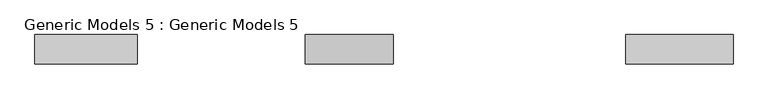
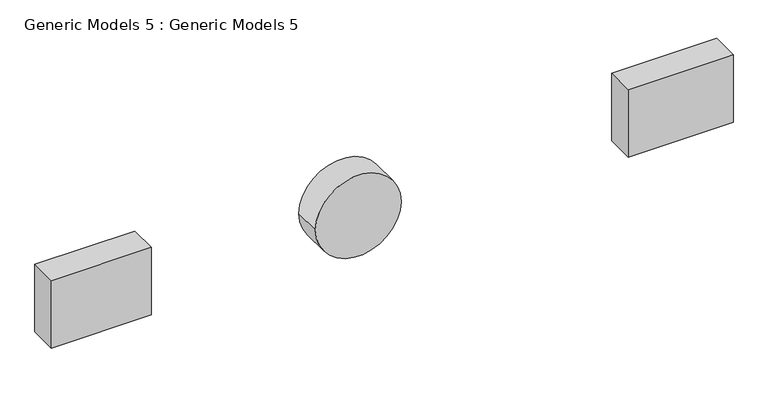
"""IFC4 building model written with IfcOpenShell, lengths in millimetres: proxy geometry, Generic Models 5 : Generic Models 5."""

from ifc_helpers import new_model, si_unit, point, frame, frame_2d, origin, place, context, project, spatial, polyline, circle_curve, trimmed, segment, composite_curve, outline, extrude, source, transform, mapped, element, save


def generic_models_5_generic_models_5_0ac3c750(model_context):
    return source(origin(), model_context, "Body", "SweptSolid", [
        extrude(outline(composite_curve([segment(trimmed(circle_curve(frame_2d((10184.7485222, -1618.2248955)), 457.2), [point((10184.7485222, -2075.4248955))], [point((10184.7485222, -1161.0248955))], False, "CARTESIAN"), True, "CONTINUOUS"), segment(trimmed(circle_curve(frame_2d((10184.7485222, -1618.2248955)), 457.2), [point((10184.7485222, -1161.0248955))], [point((10184.7485222, -2075.4248955))], False, "CARTESIAN"), True, "CONTINUOUS")], self_intersect=False)), frame((0.0, -6834.1564015, 0.0), z_axis=(0.0, 1.0, 0.0), x_axis=(0.0, 0.0, 1.0)), (0.0, 0.0, 1.0), 304.8),
        extrude(outline(polyline([(-3826.9915084, -6834.1564015), (-4893.7915084, -6834.1564015), (-4893.7915084, -6529.3564015), (-3826.9915084, -6529.3564015), (-3826.9915084, -6834.1564015)])), frame((0.0, 0.0, 9837.9470151), z_axis=(0.0, 0.0, 1.0), x_axis=(1.0, 0.0, 0.0)), (0.0, 0.0, 1.0), 762.0),
        extrude(outline(polyline([(2383.3084916, -6834.1564015), (1262.4188988, -6834.1564015), (1262.4188988, -6529.3564015), (2383.3084916, -6529.3564015), (2383.3084916, -6834.1564015)])), frame((0.0, 0.0, 9837.9470151), z_axis=(0.0, 0.0, 1.0), x_axis=(1.0, 0.0, 0.0)), (0.0, 0.0, 1.0), 762.0),
    ])


if __name__ == "__main__":
    model = new_model("IFC4")
    model_context = context("Model", 3, world=origin())
    ifc_project = project(units=[si_unit("LENGTHUNIT", "METRE", prefix="MILLI")], contexts=[model_context])
    site = spatial("IfcSite", under=ifc_project)
    building = spatial("IfcBuilding", under=site)
    placement = place(None, origin())
    generic_models_5_generic_models_5_shape = generic_models_5_generic_models_5_0ac3c750(model_context)
    element("IfcBuildingElementProxy", 1, Name="Generic Models 5 : Generic Models 5", ObjectType="Generic Models 5 : Generic Models 5", at=placement, inside=building, context=model_context, shape_type="MappedRepresentation", body=[
        mapped(generic_models_5_generic_models_5_shape, transform((0.0, 0.0, 0.0), x_axis=(1.0, 0.0, 0.0), y_axis=(0.0, 1.0, 0.0), z_axis=(0.0, 0.0, 1.0))),
    ])
    save(model, "model.ifc")

# Revit data of these elements
# Element 1 (IfcBuildingElementProxy, "Generic Models 5 : Generic Models 5")
#   Materials on its faces: "Brick, Soldier Course"
# Materials
#   "Brick, Soldier Course": class "Masonry", colour RGB 170 98 104, transparency 0, Description = "Common brick soldier coursed", Cost = 0
